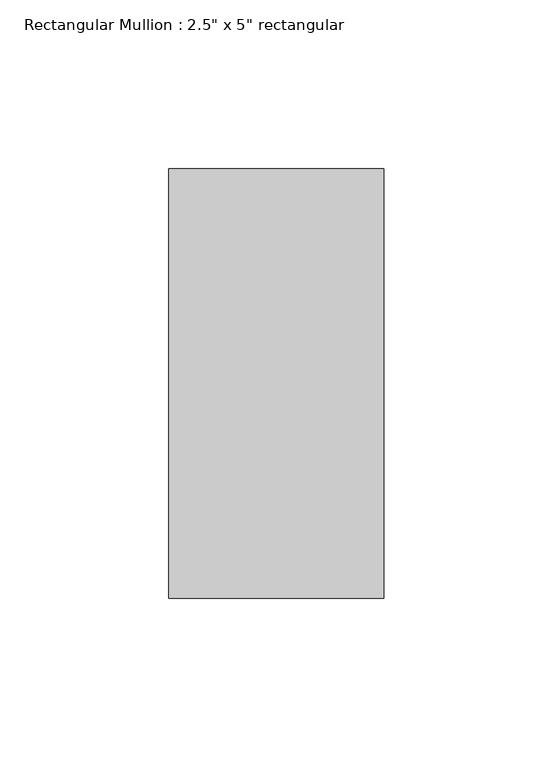
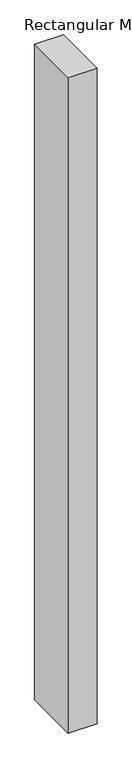
"""IFC4 building model written with IfcOpenShell, lengths in millimetres: member geometry."""

from ifc_helpers import new_model, si_unit, frame, origin, place, context, project, spatial, polyline, outline, extrude, source, transform, mapped, element, save


def member_82905deb(model_context):
    return source(origin(), model_context, "Body", "SweptSolid", [
        extrude(outline(polyline([(31.75, 63.5), (31.75, -63.5), (-31.75, -63.5), (-31.75, 63.5), (31.75, 63.5)])), frame((0.0, 0.0, -1524.0), z_axis=(0.0, 0.0, 1.0), x_axis=(1.0, 0.0, 0.0)), (0.0, 0.0, 1.0), 1524.0),
    ])


if __name__ == "__main__":
    model = new_model("IFC4")
    model_context = context("Model", 3, world=origin())
    ifc_project = project(units=[si_unit("LENGTHUNIT", "METRE", prefix="MILLI")], contexts=[model_context])
    site = spatial("IfcSite", under=ifc_project)
    building = spatial("IfcBuilding", under=site)
    placement = place(None, origin())
    member_shape = member_82905deb(model_context)
    element("IfcMember", 1, ObjectType="Rectangular Mullion : 2.5\" x 5\" rectangular", at=placement, inside=building, context=model_context, shape_type="MappedRepresentation", body=[
        mapped(member_shape, transform((0.0, 0.0, 0.0), x_axis=(1.0, 0.0, 0.0), y_axis=(0.0, 1.0, 0.0), z_axis=(0.0, 0.0, 1.0))),
    ])
    save(model, "model.ifc")

# Revit data of these elements
# Type "Rectangular Mullion : 2.5\" x 5\" rectangular"
#   built-in parameter 1007304 = 0.416667 (stored number, unit not read)
#   built-in parameter 1007301 = 0.104167 (stored number, unit not read)
#   built-in parameter 1007300 = 0.104167 (stored number, unit not read)
# Element 1 (IfcMember, "Rectangular Mullion : 2.5\" x 5\" rectangular")
#   Materials on its faces: "Rectangle 1 sq"
# Materials
#   "Rectangle 1 sq": class "Generic", colour RGB 120 120 120, transparency 0, Cost = 0
